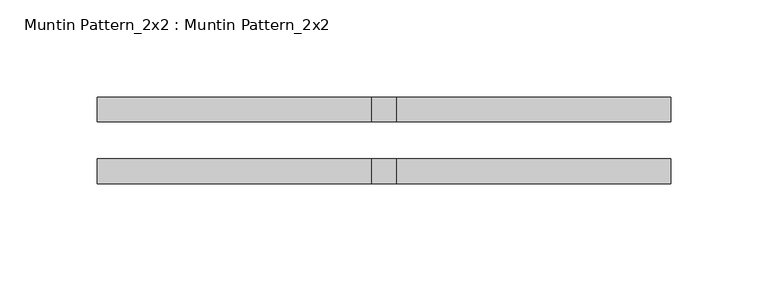
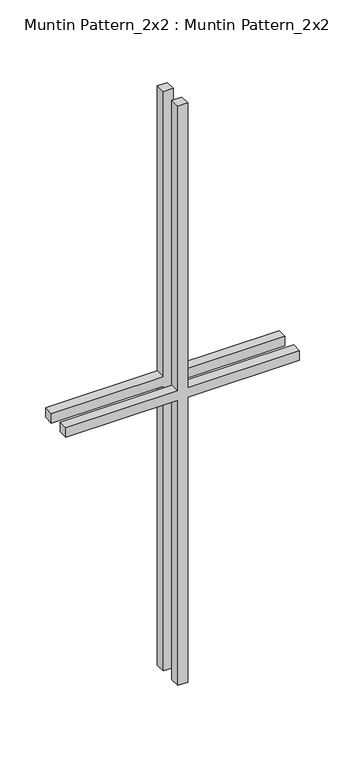
"""IFC4 building model written with IfcOpenShell, lengths in millimetres: proxy geometry, Muntin Pattern_2x2 : Muntin Pattern_2x2."""

from ifc_helpers import new_model, si_unit, frame, origin, place, context, project, spatial, polyline, outline, extrude, source, transform, mapped, element, save


def muntin_pattern_2x2_muntin_pattern_2x2_3e0ecaf2(model_context):
    return source(origin(), model_context, "Body", "SweptSolid", [
        extrude(outline(polyline([(393.7, -6.35), (393.7, -147.6375), (381.0, -147.6375), (381.0, -6.35), (0.0, -6.35), (0.0, 6.35), (381.0, 6.35), (381.0, 147.6375), (393.7, 147.6375), (393.7, 6.35), (774.7, 6.35), (774.7, -6.35), (393.7, -6.35)])), frame((0.0, -22.225, 0.0), z_axis=(0.0, 1.0, 0.0), x_axis=(0.0, 0.0, 1.0)), (0.0, 0.0, 1.0), 12.7),
        extrude(outline(polyline([(393.7, -6.35), (393.7, -147.6375), (381.0, -147.6375), (381.0, -6.35), (0.0, -6.35), (0.0, 6.35), (381.0, 6.35), (381.0, 147.6375), (393.7, 147.6375), (393.7, 6.35), (774.7, 6.35), (774.7, -6.35), (393.7, -6.35)])), frame((0.0, 9.525, 0.0), z_axis=(0.0, 1.0, 0.0), x_axis=(0.0, 0.0, 1.0)), (0.0, 0.0, 1.0), 12.7),
    ])


if __name__ == "__main__":
    model = new_model("IFC4")
    model_context = context("Model", 3, world=origin())
    ifc_project = project(units=[si_unit("LENGTHUNIT", "METRE", prefix="MILLI")], contexts=[model_context])
    site = spatial("IfcSite", under=ifc_project)
    building = spatial("IfcBuilding", under=site)
    placement = place(None, origin())
    muntin_pattern_2x2_muntin_pattern_2x2_shape = muntin_pattern_2x2_muntin_pattern_2x2_3e0ecaf2(model_context)
    element("IfcBuildingElementProxy", 1, Name="Muntin Pattern_2x2 : Muntin Pattern_2x2", ObjectType="Muntin Pattern_2x2 : Muntin Pattern_2x2", at=placement, inside=building, context=model_context, shape_type="MappedRepresentation", body=[
        mapped(muntin_pattern_2x2_muntin_pattern_2x2_shape, transform((0.0, 0.0, 0.0), x_axis=(1.0, 0.0, 0.0), y_axis=(0.0, 1.0, 0.0), z_axis=(0.0, 0.0, 1.0))),
    ])
    save(model, "model.ifc")

# Revit data of these elements
# Type "Muntin Pattern_2x2 : Muntin Pattern_2x2"
#   Width [instance default] = 48"
#   Thickness = 0.5"
#   Height [instance default] = 48"
#   Distance = 0.75"
#   Interior Material [instance default] = none
#   Exterior Material [instance default] = none
#   Default Elevation = 0
# Element 1 (IfcBuildingElementProxy, "Muntin Pattern_2x2 : Muntin Pattern_2x2")
#   Width = 11.625"
#   Height = 30.5"
#   Interior Material = Wood - Stained
#   Exterior Material = Clad - White
#   Materials on its faces: "Clad - White", "Wood - Stained"
# Materials
#   "Clad - White": class "Wood", colour RGB 242 242 238, transparency 0, Cost = 0
#   "Wood - Stained": class "Wood", colour RGB 224 178 126, transparency 0, Cost = 0
